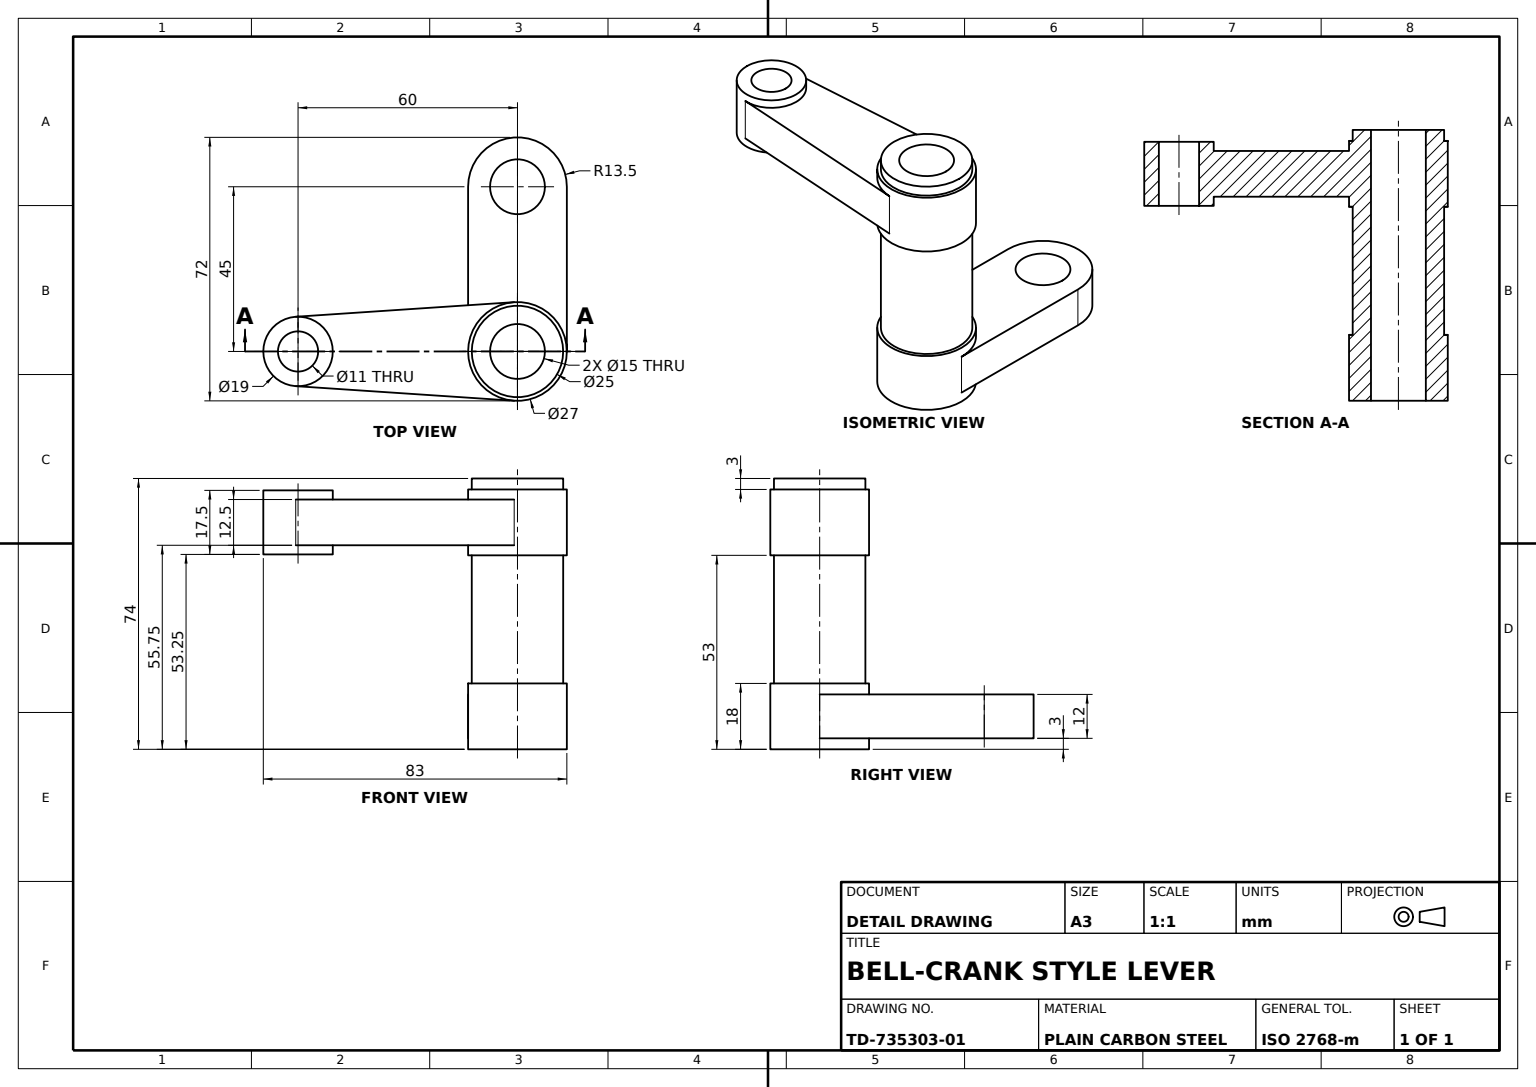
SolidWorks part; units mm, degrees
material "Plain Carbon Steel"
ref_plane "Front Plane" through (0, 0, 0) normal (0, 0, 1) x (1, 0, 0)
ref_plane "Top Plane" through (0, 0, 0) normal (0, 1, 0) x (1, 0, 0)
ref_plane "Right Plane" through (0, 0, 0) normal (1, 0, 0) x (0, 0, -1)
sketch "Lower Arm Sketch" plane through (0, 0, 0) normal (0, 1, 0) x (1, 0, 0)
  line L0 (0, 0) -> (-45, 0) construction
  line L1 (-45, 13.5) -> (0, 13.5)
  line L2 (-45, -13.5) -> (0, -13.5)
  arc A0 (0, -13.5) -> (0, 13.5) centre (0, 0) ccw
  arc A1 (-45, 13.5) -> (-45, -13.5) centre (-45, 0) ccw
  circle A2 centre (-45, 0) radius 7.5
  dimension "D1" = 27
  dimension "D2" = 27
  dimension "D4" = 15
  dimension "D3" = 45
extrude "Lower Arm" add sketch "Lower Arm Sketch" along normal mid plane 12
sketch "Hub Base Sketch" plane through (0, 0, 0) normal (0, 1, 0) x (1, 0, 0)
  circle A0 centre (0, 0) radius 13.5
  dimension "D1" = 27
extrude "Hub Base Boss" add sketch "Hub Base Sketch" along normal mid plane 18
sketch "Pivot Hub Profile" plane through (0, 0, 0) normal (0, 0, 1) x (1, 0, 0)
  line L0 (0, 0) -> (0, 65)
  line L1 (0, 65) -> (12.5, 65)
  line L2 (12.5, 65) -> (12.5, 62)
  line L3 (12.5, 62) -> (13.5, 62)
  line L4 (13.5, 62) -> (13.5, 44)
  line L5 (13.5, 44) -> (12.5, 44)
  line L6 (12.5, 44) -> (12.5, 0)
  line L7 (12.5, 0) -> (0, 0)
  line L8 (-13.5, -9) -> (13.5, -9) construction
  line L9 (13.5, -9) -> (13.5, 9) construction
  dimension "D1" = 3
  dimension "D2" = 74
  dimension "D3" = 18
  dimension "D4" = 12.5
revolve "Pivot Hub" add sketch "Pivot Hub Profile" angle 360 about L0
sketch "Pivot Bore Sketch" plane through (0, 65, 0) normal (0, 1, 0) x (1, 0, 0)
  circle A0 centre (0, 0) radius 7.5
  dimension "D1" = 15
extrude "Pivot Bore Ø15" cut sketch "Pivot Bore Sketch" against normal through all
ref_plane "Upper Arm Plane" through (0, 53, 0) normal (0, 1, 0) x (1, 0, 0)
sketch "End Boss Sketch" plane through (0, 53, 0) normal (0, 1, 0) x (1, 0, 0)
  circle A0 centre (0, -60) radius 9.5
  circle A1 centre (0, -60) radius 5.5
  dimension "D1" = 19
  dimension "D2" = 11
  dimension "D3" = 60
extrude "End Boss Ø19" add sketch "End Boss Sketch" along normal mid plane 17.5 separate body
sketch "Upper Arm Sketch" plane through (0, 53, 0) normal (0, 1, 0) x (1, 0, 0)
  line L0 (13.47, -0.9) -> (9.4789, -60.6333)
  line L1 (0, 0) -> (0, -33.5637) construction
  line L2 (-13.47, -0.9) -> (-9.4789, -60.6333)
  circle A0 centre (0, 0) radius 13.5 construction
  circle A1 centre (0, -60) radius 9.5 construction
  arc A2 (-13.47, -0.9) -> (13.47, -0.9) centre (0, 0) ccw
  arc A3 (9.4789, -60.6333) -> (-9.4789, -60.6333) centre (0, -60) ccw
extrude "Upper Arm" add sketch "Upper Arm Sketch" along normal mid plane 12.5
